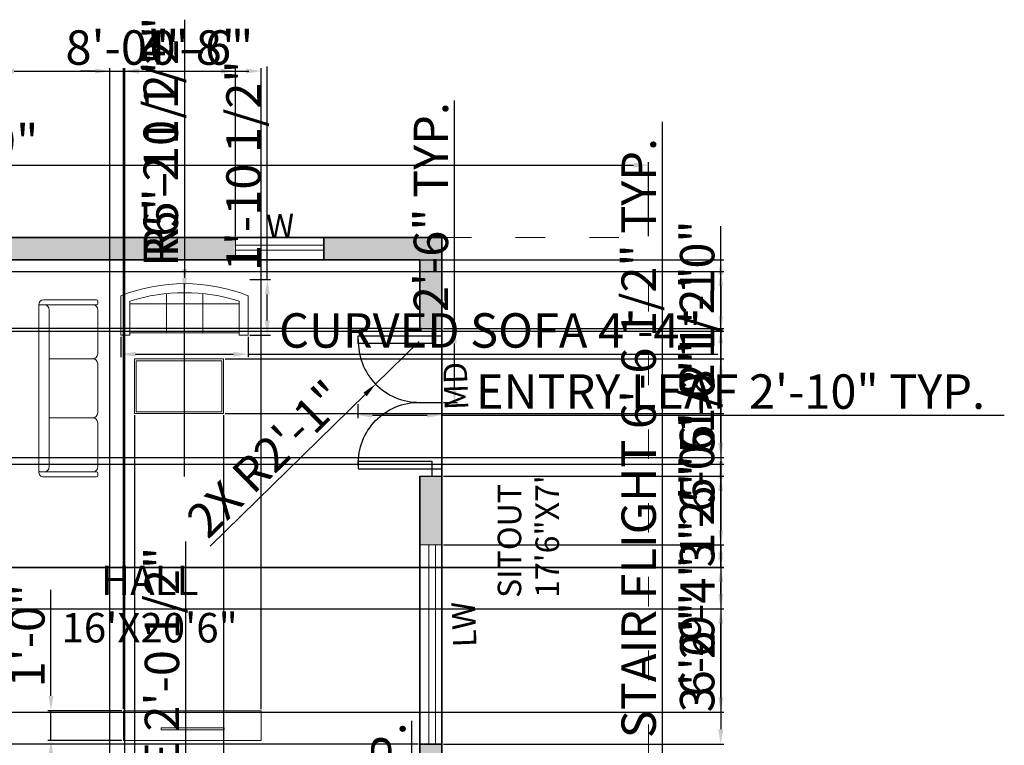
# Model space of a CAD drawing. Units: inches. Extents: x 2961 to 3748, y 1432 to 1961.
# Tile 9 of 9: x 3348 to 3748, y 1658 to 1953. Entities that reach past the tile are written whole.
import ezdxf
from ezdxf.enums import TextEntityAlignment as Align

# ---------------------------------------------------------------- set-up
doc = ezdxf.new("R2010")
doc.units = ezdxf.units.IN
doc.linetypes.add('ACAD_ISO03W100', pattern=[30, 12, -18])
for name, color, linetype, lineweight in [('A-ANNO-DIMS', 2, 'Continuous', 18), ('A-ANNO-TEXT', 7, 'Continuous', 18), ('A-AREA-IDEN', 7, 'Continuous', 18), ('A-DOOR', 3, 'Continuous', 25), ('A-FURN', 8, 'Continuous', 18), ('A-GLAZ', 4, 'Continuous', 18), ('A-ROOF-OVHD', 8, 'ACAD_ISO03W100', 18), ('A-WALL', 7, 'Continuous', 35), ('A-WALL-PATT', 252, 'Continuous', 13)]:
    doc.layers.add(name, color=color, linetype=linetype, lineweight=lineweight)
doc.styles.get("Standard").update_dxf_attribs({"font": 'arial.ttf'})
doc.dimstyles.new('ISO-25', dxfattribs={"dimtxt": 14, "dimasz": 6, "dimexe": 1.25, "dimexo": 0.625, "dimtad": 1, "dimlunit": 3, "dimtxsty": 'Standard', "dimcen": 2.5, "dimadec": 0, "dimazin": 0, "dimtfac": 1, "dimtmove": 0, "dimatfit": 3, "dimfxl": 1, "dimarcsym": 0})

# ---------------------------------------------------------------- blocks, each defined once
blk = doc.blocks.new('sofa')
for p, q in [((1024.17, 311.16), (1024.17, 289.66)), ((1024.67, 311.66), (1025.67, 311.66)), ((1026.17, 308), (1026.17, 311.16)), ((1048.17, 309.66), (1048.17, 291.87)), ((1048.17, 309.66), (1048.17, 309.66)), ((1050.17, 311.66), (1070.17, 311.66)), ((1072.17, 309.66), (1072.17, 291.87)), ((1072.17, 309.66), (1072.17, 309.66)), ((1094.17, 309.66), (1094.17, 311.16)), ((1095.67, 311.66), (1094.67, 311.66)), ((1096.17, 289.66), (1096.17, 311.16)), ((1026.17, 287.66), (1094.17, 287.66))]:
    blk.add_line(p, q)
for points in [[(1046.17, 311.66), (1028.17, 311.66, 0.414214), (1026.17, 309.66), (1026.17, 288.16)], [(1074.17, 311.66), (1092.17, 311.66, -0.414214), (1094.17, 309.66), (1094.17, 288.16)]]:
    blk.add_lwpolyline(points, format="xyb")
blk.add_lwpolyline([(1026.67, 287.66), (1093.67, 287.66, 0.414214), (1094.17, 288.16), (1094.17, 289.87, 0.414214), (1092.17, 291.87), (1028.17, 291.87, 0.414214), (1026.17, 289.87), (1026.17, 288.16, 0.414214)], format="xyb", close=True)
for centre, radius, start, end in [((1024.67, 311.16), 0.5, 90, 180), ((1025.67, 311.16), 0.5, 0, 90), ((1046.17, 309.66), 2, 0, 90), ((1050.17, 309.66), 2, 90, 180), ((1070.17, 309.66), 2, 0, 90), ((1074.17, 309.66), 2, 90, 180), ((1094.67, 311.16), 0.5, 90, 180), ((1095.67, 311.16), 0.5, 0, 90), ((1026.17, 289.66), 2, 180, 270), ((1094.17, 289.66), 2, 270, 0)]:
    blk.add_arc(centre, radius, start, end)
blk = doc.blocks.new('Sofa - Roundback 7 ft.')
for p, q in [((-36.000027, -34), (-36.000027, -11.4696)), ((-12.00002, -32.4421), (-12.00003, -6.5971)), ((11.99997, -32.4421), (11.99998, -6.5971)), ((35.99998, -34), (35.99998, -11.4696)), ((-35.999844, -13.3819), (35.9998, -13.3819)), ((-36.000027, -32.4421), (35.99998, -32.4421))]:
    blk.add_line(p, q)
for points in [[(-36.000027, -34), (-42.000027, -34), (-42.000027, -8)], [(41.99998, -8), (41.99998, -34), (35.99998, -34)]]:
    blk.add_lwpolyline(points)
for centre, radius, start, end in [((0, -114.25), 114.25, 68.43141, 111.5686), ((-0.00001, -127.1968), 121.1968, 72.72033, 107.2797)]:
    blk.add_arc(centre, radius, start, end)
blk = doc.blocks.new('*D14')
at = {"layer": 'A-ANNO-DIMS', "color": 0, "lineweight": -2, "transparency": 16777216}
for p, q in [((3054.27, 1865.26), (3054.27, 1895.31)), ((3603.27, 1865.26), (3603.27, 1895.31)), ((3060.27, 1894.06), (3597.27, 1894.06))]:
    blk.add_line(p, q, dxfattribs=at)
at = {"layer": 'A-ANNO-DIMS', "color": 0, "transparency": 16777216}
for points in [[(3060.27, 1895.06), (3060.27, 1893.06), (3054.27, 1894.06)], [(3597.27, 1895.06), (3597.27, 1893.06), (3603.27, 1894.06)]]:
    blk.add_solid(points, dxfattribs=at)
at = {"layer": 'Defpoints', "color": 0, "transparency": 16777216}
for p in [(3603.27, 1894.06), (3054.27, 1864.64), (3603.27, 1864.64)]:
    blk.add_point(p, dxfattribs=at)
at = {"layer": 'A-ANNO-DIMS', "color": 0, "transparency": 16777216, "insert": (3328.77, 1901.84), "char_height": 14, "attachment_point": 5}
blk.add_mtext('45\'-9"', dxfattribs=at)
blk = doc.blocks.new('WIN-36IN')
for p, q in [((0, 6), (36, 6)), ((0, 3.9), (36, 3.9))]:
    blk.add_line(p, q)
blk.add_lwpolyline([(36, 9), (0, 9), (0, 0), (36, 0)], close=True)
blk = doc.blocks.new('DOOR-ENTRY-LEAF-30IN')
for p, q in [((25, 30), (34, 30)), ((30, 30), (30, 27)), ((30, 27), (34, 27))]:
    blk.add_line(p, q)
blk.add_lwpolyline([(30, 27), (30, 24), (0, 24), (0, 27)], close=True)
blk.add_arc((24.74, 24.75), 24.75, 178.2636, 270.6019)
blk = doc.blocks.new('*D32')
at = {"layer": 'A-ANNO-DIMS', "color": 0, "lineweight": -2, "transparency": 16777216}
for p, q in [((3485.06, 1796.94), (3485.06, 1791.19)), ((3519.27, 1796.94), (3519.27, 1791.19)), ((3491.06, 1792.44), (3513.27, 1792.44)), ((3519.27, 1792.44), (3748.06, 1792.44))]:
    blk.add_line(p, q, dxfattribs=at)
at = {"layer": 'A-ANNO-DIMS', "color": 0, "transparency": 16777216}
for points in [[(3491.06, 1793.44), (3491.06, 1791.44), (3485.06, 1792.44)], [(3513.27, 1793.44), (3513.27, 1791.44), (3519.27, 1792.44)]]:
    blk.add_solid(points, dxfattribs=at)
at = {"layer": 'Defpoints', "color": 0, "transparency": 16777216}
for p in [(3485.06, 1797.57), (3519.27, 1797.57), (3519.27, 1792.44)]:
    blk.add_point(p, dxfattribs=at)
at = {"layer": 'A-ANNO-DIMS', "color": 0, "transparency": 16777216, "insert": (3636.66, 1800.21), "char_height": 14, "attachment_point": 5}
blk.add_mtext('ENTRY LEAF 2\'-10" TYP.', dxfattribs=at)
blk = doc.blocks.new('*D33')
at = {"layer": 'A-ANNO-DIMS', "color": 0, "lineweight": -2, "transparency": 16777216}
for p, q in [((3524.4, 1827.64), (3524.4, 1920.46)), ((3519.89, 1827.64), (3525.65, 1827.64)), ((3524.4, 1803.57), (3524.4, 1821.64)), ((3519.89, 1797.57), (3525.65, 1797.57))]:
    blk.add_line(p, q, dxfattribs=at)
at = {"layer": 'A-ANNO-DIMS', "color": 0, "transparency": 16777216}
for points in [[(3523.4, 1821.64), (3525.4, 1821.64), (3524.4, 1827.64)], [(3523.4, 1803.57), (3525.4, 1803.57), (3524.4, 1797.57)]]:
    blk.add_solid(points, dxfattribs=at)
at = {"layer": 'Defpoints', "color": 0, "transparency": 16777216}
for p in [(3519.27, 1827.64), (3524.4, 1827.64), (3519.27, 1797.57)]:
    blk.add_point(p, dxfattribs=at)
at = {"layer": 'A-ANNO-DIMS', "color": 0, "transparency": 16777216, "insert": (3516.62, 1877.05), "char_height": 14, "attachment_point": 5, "rotation": 90}
blk.add_mtext('2\'-6" TYP.', dxfattribs=at)
blk = doc.blocks.new('*D35')
at = {"layer": 'A-ANNO-DIMS', "color": 0, "lineweight": -2, "transparency": 16777216}
for p, q in [((3507, 1575.49), (3507, 1668.08)), ((3506.23, 1569.49), (3508.25, 1569.49)), ((3507, 1560.25), (3507, 1569.49)), ((3506.23, 1560.25), (3508.25, 1560.25)), ((3507, 1554.25), (3507, 1548.25))]:
    blk.add_line(p, q, dxfattribs=at)
at = {"layer": 'A-ANNO-DIMS', "color": 0, "transparency": 16777216}
for points in [[(3506, 1575.49), (3508, 1575.49), (3507, 1569.49)], [(3506, 1554.25), (3508, 1554.25), (3507, 1560.25)]]:
    blk.add_solid(points, dxfattribs=at)
at = {"layer": 'Defpoints', "color": 0, "transparency": 16777216}
for p in [(3505.61, 1569.49), (3507, 1569.49), (3505.61, 1560.25)]:
    blk.add_point(p, dxfattribs=at)
at = {"layer": 'A-ANNO-DIMS', "color": 0, "transparency": 16777216, "insert": (3499.22, 1624.78), "char_height": 14, "attachment_point": 5, "rotation": 90}
blk.add_mtext('0\'-9" TYP.', dxfattribs=at)
blk = doc.blocks.new('*D36')
at = {"layer": 'A-ANNO-DIMS', "color": 0, "lineweight": -2, "transparency": 16777216}
for p, q in [((3609.01, 1648.54), (3609.01, 1911.68)), ((3597.89, 1648.54), (3610.26, 1648.54)), ((3609.01, 1576.24), (3609.01, 1642.54)), ((3597.89, 1570.24), (3610.26, 1570.24))]:
    blk.add_line(p, q, dxfattribs=at)
at = {"layer": 'A-ANNO-DIMS', "color": 0, "transparency": 16777216}
for points in [[(3608.01, 1642.54), (3610.01, 1642.54), (3609.01, 1648.54)], [(3608.01, 1576.24), (3610.01, 1576.24), (3609.01, 1570.24)]]:
    blk.add_solid(points, dxfattribs=at)
at = {"layer": 'Defpoints', "color": 0, "transparency": 16777216}
for p in [(3597.27, 1648.54), (3609.01, 1648.54), (3597.27, 1570.24)]:
    blk.add_point(p, dxfattribs=at)
at = {"layer": 'A-ANNO-DIMS', "color": 0, "transparency": 16777216, "insert": (3601.15, 1783.11), "char_height": 14, "attachment_point": 5, "rotation": 90}
blk.add_mtext('STAIR FLIGHT 6\'-6 1/2" TYP.', dxfattribs=at)
blk = doc.blocks.new('*D40')
at = {"layer": 'A-ANNO-DIMS', "color": 0, "lineweight": -2, "transparency": 16777216}
for p, q in [((3415.09, 1585.45), (3415.09, 1741.07)), ((3412.07, 1585.45), (3416.34, 1585.45)), ((3415.09, 1567.11), (3415.09, 1579.45)), ((3412.07, 1561.11), (3416.34, 1561.11))]:
    blk.add_line(p, q, dxfattribs=at)
at = {"layer": 'A-ANNO-DIMS', "color": 0, "transparency": 16777216}
for points in [[(3414.09, 1579.45), (3416.09, 1579.45), (3415.09, 1585.45)], [(3414.09, 1567.11), (3416.09, 1567.11), (3415.09, 1561.11)]]:
    blk.add_solid(points, dxfattribs=at)
at = {"layer": 'Defpoints', "color": 0, "transparency": 16777216}
for p in [(3411.44, 1585.45), (3415.09, 1585.45), (3411.44, 1561.11)]:
    blk.add_point(p, dxfattribs=at)
at = {"layer": 'A-ANNO-DIMS', "color": 0, "transparency": 16777216, "insert": (3407.23, 1666.26), "char_height": 14, "attachment_point": 5, "rotation": 90}
blk.add_mtext('FRIDGE 2\'-0 1/2"', dxfattribs=at)
blk = doc.blocks.new('*D48')
at = {"layer": 'A-ANNO-DIMS', "color": 0, "lineweight": -2, "transparency": 16777216}
for p, q in [((3388.72, 1824.34), (3388.72, 1815.95)), ((3440.5, 1824.34), (3440.5, 1815.95)), ((3394.72, 1817.2), (3434.5, 1817.2)), ((3440.5, 1817.2), (3631.5, 1817.2))]:
    blk.add_line(p, q, dxfattribs=at)
at = {"layer": 'A-ANNO-DIMS', "color": 0, "transparency": 16777216}
for points in [[(3394.72, 1818.2), (3394.72, 1816.2), (3388.72, 1817.2)], [(3434.5, 1818.2), (3434.5, 1816.2), (3440.5, 1817.2)]]:
    blk.add_solid(points, dxfattribs=at)
at = {"layer": 'Defpoints', "color": 0, "transparency": 16777216}
for p in [(3388.72, 1824.96), (3440.5, 1824.96), (3440.5, 1817.2)]:
    blk.add_point(p, dxfattribs=at)
at = {"layer": 'A-ANNO-DIMS', "color": 0, "transparency": 16777216, "insert": (3539, 1825.07), "char_height": 14, "attachment_point": 5}
blk.add_mtext('CURVED SOFA 4\'-4"', dxfattribs=at)
blk = doc.blocks.new('*D49')
at = {"layer": 'A-ANNO-DIMS', "color": 0, "lineweight": -2, "transparency": 16777216}
for p, q in [((3448.26, 1847.57), (3448.26, 1934.21)), ((3441.12, 1847.57), (3449.51, 1847.57)), ((3448.26, 1830.96), (3448.26, 1841.57)), ((3441.12, 1824.96), (3449.51, 1824.96))]:
    blk.add_line(p, q, dxfattribs=at)
at = {"layer": 'A-ANNO-DIMS', "color": 0, "transparency": 16777216}
for points in [[(3447.26, 1841.57), (3449.26, 1841.57), (3448.26, 1847.57)], [(3447.26, 1830.96), (3449.26, 1830.96), (3448.26, 1824.96)]]:
    blk.add_solid(points, dxfattribs=at)
at = {"layer": 'Defpoints', "color": 0, "transparency": 16777216}
for p in [(3440.5, 1847.57), (3448.26, 1847.57), (3440.5, 1824.96)]:
    blk.add_point(p, dxfattribs=at)
at = {"layer": 'A-ANNO-DIMS', "color": 0, "transparency": 16777216, "insert": (3440.4, 1893.89), "char_height": 14, "attachment_point": 5, "rotation": 90}
blk.add_mtext('1\'-10 1/2"', dxfattribs=at)
blk = doc.blocks.new('*D52')
at = {"layer": 'A-ANNO-DIMS', "color": 0, "lineweight": -2, "transparency": 16777216}
for p, q in [((3360.27, 1678.21), (3360.27, 1721.36)), ((3389.1, 1672.21), (3359.02, 1672.21)), ((3360.27, 1660.05), (3360.27, 1672.21)), ((3389.1, 1660.05), (3359.02, 1660.05)), ((3360.27, 1654.05), (3360.27, 1648.05))]:
    blk.add_line(p, q, dxfattribs=at)
at = {"layer": 'A-ANNO-DIMS', "color": 0, "transparency": 16777216}
for points in [[(3359.27, 1678.21), (3361.27, 1678.21), (3360.27, 1672.21)], [(3359.27, 1654.05), (3361.27, 1654.05), (3360.27, 1660.05)]]:
    blk.add_solid(points, dxfattribs=at)
at = {"layer": 'Defpoints', "color": 0, "transparency": 16777216}
for p in [(3360.27, 1672.21), (3389.72, 1672.21), (3389.72, 1660.05)]:
    blk.add_point(p, dxfattribs=at)
at = {"layer": 'A-ANNO-DIMS', "color": 0, "transparency": 16777216, "insert": (3352.5, 1702.78), "char_height": 14, "attachment_point": 5, "rotation": 90}
blk.add_mtext('1\'-0"', dxfattribs=at)
blk = doc.blocks.new('*D55')
at = {"layer": 'A-ANNO-DIMS', "color": 0, "lineweight": -2, "transparency": 16777216}
for p, q in [((3339.27, 1865.26), (3339.27, 1933.63)), ((3345.27, 1932.38), (3429.27, 1932.38)), ((3435.27, 1865.26), (3435.27, 1933.63))]:
    blk.add_line(p, q, dxfattribs=at)
at = {"layer": 'A-ANNO-DIMS', "color": 0, "transparency": 16777216}
for points in [[(3345.27, 1933.38), (3345.27, 1931.38), (3339.27, 1932.38)], [(3429.27, 1933.38), (3429.27, 1931.38), (3435.27, 1932.38)]]:
    blk.add_solid(points, dxfattribs=at)
at = {"layer": 'Defpoints', "color": 0, "transparency": 16777216}
for p in [(3435.27, 1932.38), (3339.27, 1864.64), (3435.27, 1864.64)]:
    blk.add_point(p, dxfattribs=at)
at = {"layer": 'A-ANNO-DIMS', "color": 0, "transparency": 16777216, "insert": (3387.27, 1940.15), "char_height": 14, "attachment_point": 5}
blk.add_mtext('8\'-0"', dxfattribs=at)
blk = doc.blocks.new('*D64')
at = {"layer": 'A-ANNO-DIMS', "color": 0, "lineweight": -2, "transparency": 16777216}
for p, q in [((3509.64, 1855.64), (3023.57, 1855.64)), ((3024.82, 1849.64), (3024.82, 1833.64)), ((3509.64, 1827.64), (3023.57, 1827.64)), ((3024.82, 1827.64), (3024.82, 1782.93))]:
    blk.add_line(p, q, dxfattribs=at)
at = {"layer": 'A-ANNO-DIMS', "color": 0, "transparency": 16777216}
for points in [[(3023.82, 1849.64), (3025.82, 1849.64), (3024.82, 1855.64)], [(3023.82, 1833.64), (3025.82, 1833.64), (3024.82, 1827.64)]]:
    blk.add_solid(points, dxfattribs=at)
at = {"layer": 'Defpoints', "color": 0, "transparency": 16777216}
for p in [(3510.27, 1855.64), (3024.82, 1827.64), (3510.27, 1827.64)]:
    blk.add_point(p, dxfattribs=at)
at = {"layer": 'A-ANNO-DIMS', "color": 0, "transparency": 16777216, "insert": (3017.16, 1802.29), "char_height": 14, "attachment_point": 5, "rotation": 90}
blk.add_mtext('2\'-4"', dxfattribs=at)
blk = doc.blocks.new('*D65')
at = {"layer": 'A-ANNO-DIMS', "color": 0, "lineweight": -2, "transparency": 16777216}
for p, q in [((3519.89, 1827.64), (3633.97, 1827.64)), ((3632.72, 1821.64), (3632.72, 1773.64)), ((3519.89, 1767.64), (3633.97, 1767.64))]:
    blk.add_line(p, q, dxfattribs=at)
at = {"layer": 'A-ANNO-DIMS', "color": 0, "transparency": 16777216}
for points in [[(3631.72, 1821.64), (3633.72, 1821.64), (3632.72, 1827.64)], [(3631.72, 1773.64), (3633.72, 1773.64), (3632.72, 1767.64)]]:
    blk.add_solid(points, dxfattribs=at)
at = {"layer": 'Defpoints', "color": 0, "transparency": 16777216}
for p in [(3519.27, 1827.64), (3519.27, 1767.64), (3632.72, 1767.64)]:
    blk.add_point(p, dxfattribs=at)
at = {"layer": 'A-ANNO-DIMS', "color": 0, "transparency": 16777216, "insert": (3624.94, 1797.64), "char_height": 14, "attachment_point": 5, "rotation": 90}
blk.add_mtext('5\'-0"', dxfattribs=at)
blk = doc.blocks.new('*D66')
at = {"layer": 'A-ANNO-DIMS', "color": 0, "lineweight": -2, "transparency": 16777216}
for p, q in [((3519.89, 1767.64), (3633.97, 1767.64)), ((3632.72, 1761.64), (3632.72, 1745.64)), ((3519.89, 1739.64), (3633.97, 1739.64)), ((3632.72, 1739.64), (3632.72, 1694.93))]:
    blk.add_line(p, q, dxfattribs=at)
at = {"layer": 'A-ANNO-DIMS', "color": 0, "transparency": 16777216}
for points in [[(3631.72, 1761.64), (3633.72, 1761.64), (3632.72, 1767.64)], [(3631.72, 1745.64), (3633.72, 1745.64), (3632.72, 1739.64)]]:
    blk.add_solid(points, dxfattribs=at)
at = {"layer": 'Defpoints', "color": 0, "transparency": 16777216}
for p in [(3519.27, 1767.64), (3519.27, 1739.64), (3632.72, 1739.64)]:
    blk.add_point(p, dxfattribs=at)
at = {"layer": 'A-ANNO-DIMS', "color": 0, "transparency": 16777216, "insert": (3625.06, 1714.29), "char_height": 14, "attachment_point": 5, "rotation": 90}
blk.add_mtext('2\'-4"', dxfattribs=at)
blk = doc.blocks.new('*D67')
at = {"layer": 'A-ANNO-DIMS', "color": 0, "lineweight": -2, "transparency": 16777216}
for p, q in [((3519.89, 1739.64), (3633.97, 1739.64)), ((3632.72, 1733.64), (3632.72, 1664.64)), ((3519.89, 1658.64), (3633.97, 1658.64))]:
    blk.add_line(p, q, dxfattribs=at)
at = {"layer": 'A-ANNO-DIMS', "color": 0, "transparency": 16777216}
for points in [[(3631.72, 1733.64), (3633.72, 1733.64), (3632.72, 1739.64)], [(3631.72, 1664.64), (3633.72, 1664.64), (3632.72, 1658.64)]]:
    blk.add_solid(points, dxfattribs=at)
at = {"layer": 'Defpoints', "color": 0, "transparency": 16777216}
for p in [(3519.27, 1739.64), (3519.27, 1658.64), (3632.72, 1658.64)]:
    blk.add_point(p, dxfattribs=at)
at = {"layer": 'A-ANNO-DIMS', "color": 0, "transparency": 16777216, "insert": (3624.94, 1699.14), "char_height": 14, "attachment_point": 5, "rotation": 90}
blk.add_mtext('6\'-9"', dxfattribs=at)
blk = doc.blocks.new('*D68')
at = {"layer": 'A-ANNO-DIMS', "color": 0, "lineweight": -2, "transparency": 16777216}
for p, q in [((3024.82, 1658.64), (3024.82, 1701.79)), ((3509.64, 1658.64), (3023.57, 1658.64)), ((3024.82, 1647.64), (3024.82, 1652.64)), ((3509.64, 1641.64), (3023.57, 1641.64))]:
    blk.add_line(p, q, dxfattribs=at)
at = {"layer": 'A-ANNO-DIMS', "color": 0, "transparency": 16777216}
for points in [[(3023.82, 1652.64), (3025.82, 1652.64), (3024.82, 1658.64)], [(3023.82, 1647.64), (3025.82, 1647.64), (3024.82, 1641.64)]]:
    blk.add_solid(points, dxfattribs=at)
at = {"layer": 'Defpoints', "color": 0, "transparency": 16777216}
for p in [(3024.82, 1658.64), (3510.27, 1658.64), (3510.27, 1641.64)]:
    blk.add_point(p, dxfattribs=at)
at = {"layer": 'A-ANNO-DIMS', "color": 0, "transparency": 16777216, "insert": (3017.04, 1683.21), "char_height": 14, "attachment_point": 5, "rotation": 90}
blk.add_mtext('1\'-5"', dxfattribs=at)
blk = doc.blocks.new('*D70')
at = {"layer": 'A-ANNO-DIMS', "color": 0, "lineweight": -2, "transparency": 16777216}
for p, q in [((3024.82, 1641.64), (3024.82, 1686.09)), ((3383.64, 1641.64), (3023.57, 1641.64)), ((3024.82, 1611.64), (3024.82, 1635.64)), ((3383.64, 1605.64), (3023.57, 1605.64))]:
    blk.add_line(p, q, dxfattribs=at)
at = {"layer": 'A-ANNO-DIMS', "color": 0, "transparency": 16777216}
for points in [[(3023.82, 1635.64), (3025.82, 1635.64), (3024.82, 1641.64)], [(3023.82, 1611.64), (3025.82, 1611.64), (3024.82, 1605.64)]]:
    blk.add_solid(points, dxfattribs=at)
at = {"layer": 'Defpoints', "color": 0, "transparency": 16777216}
for p in [(3024.82, 1641.64), (3384.27, 1641.64), (3384.27, 1605.64)]:
    blk.add_point(p, dxfattribs=at)
at = {"layer": 'A-ANNO-DIMS', "color": 0, "transparency": 16777216, "insert": (3017.04, 1666.87), "char_height": 14, "attachment_point": 5, "rotation": 90}
blk.add_mtext('3\'-0"', dxfattribs=at)
blk = doc.blocks.new('*D71')
at = {"layer": 'A-ANNO-DIMS', "color": 0, "lineweight": -2, "transparency": 16777216}
for p, q in [((3255.89, 1772.53), (3633.97, 1772.53)), ((3632.72, 1736.64), (3632.72, 1766.53)), ((3255.89, 1730.64), (3633.97, 1730.64))]:
    blk.add_line(p, q, dxfattribs=at)
at = {"layer": 'A-ANNO-DIMS', "color": 0, "transparency": 16777216}
for points in [[(3631.72, 1766.53), (3633.72, 1766.53), (3632.72, 1772.53)], [(3631.72, 1736.64), (3633.72, 1736.64), (3632.72, 1730.64)]]:
    blk.add_solid(points, dxfattribs=at)
at = {"layer": 'Defpoints', "color": 0, "transparency": 16777216}
for p in [(3255.27, 1772.53), (3632.72, 1772.53), (3255.27, 1730.64)]:
    blk.add_point(p, dxfattribs=at)
at = {"layer": 'A-ANNO-DIMS', "color": 0, "transparency": 16777216, "insert": (3624.94, 1751.59), "char_height": 14, "attachment_point": 5, "rotation": 90}
blk.add_mtext('3\'-6"', dxfattribs=at)
blk = doc.blocks.new('*D72')
at = {"layer": 'A-ANNO-DIMS', "color": 0, "lineweight": -2, "transparency": 16777216}
for p, q in [((3255.89, 1713.64), (3633.97, 1713.64)), ((3632.72, 1677.64), (3632.72, 1707.64)), ((3255.89, 1671.64), (3633.97, 1671.64))]:
    blk.add_line(p, q, dxfattribs=at)
at = {"layer": 'A-ANNO-DIMS', "color": 0, "transparency": 16777216}
for points in [[(3631.72, 1707.64), (3633.72, 1707.64), (3632.72, 1713.64)], [(3631.72, 1677.64), (3633.72, 1677.64), (3632.72, 1671.64)]]:
    blk.add_solid(points, dxfattribs=at)
at = {"layer": 'Defpoints', "color": 0, "transparency": 16777216}
for p in [(3255.27, 1713.64), (3632.72, 1713.64), (3255.27, 1671.64)]:
    blk.add_point(p, dxfattribs=at)
at = {"layer": 'A-ANNO-DIMS', "color": 0, "transparency": 16777216, "insert": (3624.94, 1692.64), "char_height": 14, "attachment_point": 5, "rotation": 90}
blk.add_mtext('3\'-6"', dxfattribs=at)
blk = doc.blocks.new('*D76')
at = {"layer": 'A-ANNO-DIMS', "color": 0, "lineweight": -2, "transparency": 16777216}
for p, q in [((3632.72, 1730.53), (3632.72, 1773.68)), ((3264.89, 1730.53), (3633.97, 1730.53)), ((3632.72, 1719.64), (3632.72, 1724.53)), ((3264.89, 1713.64), (3633.97, 1713.64))]:
    blk.add_line(p, q, dxfattribs=at)
at = {"layer": 'A-ANNO-DIMS', "color": 0, "transparency": 16777216}
for points in [[(3631.72, 1724.53), (3633.72, 1724.53), (3632.72, 1730.53)], [(3631.72, 1719.64), (3633.72, 1719.64), (3632.72, 1713.64)]]:
    blk.add_solid(points, dxfattribs=at)
at = {"layer": 'Defpoints', "color": 0, "transparency": 16777216}
for p in [(3264.27, 1730.53), (3632.72, 1730.53), (3264.27, 1713.64)]:
    blk.add_point(p, dxfattribs=at)
at = {"layer": 'A-ANNO-DIMS', "color": 0, "transparency": 16777216, "insert": (3624.94, 1755.11), "char_height": 14, "attachment_point": 5, "rotation": 90}
blk.add_mtext('1\'-5"', dxfattribs=at)
blk = doc.blocks.new('*D78')
at = {"layer": 'A-ANNO-DIMS', "color": 0, "lineweight": -2, "transparency": 16777216}
for p, q in [((3394.23, 1792.44), (3394.23, 1473.94)), ((3430.5, 1792.44), (3430.5, 1473.94)), ((3400.23, 1475.19), (3424.5, 1475.19)), ((3430.5, 1475.19), (3507.58, 1475.19))]:
    blk.add_line(p, q, dxfattribs=at)
at = {"layer": 'A-ANNO-DIMS', "color": 0, "transparency": 16777216}
for points in [[(3400.23, 1476.19), (3400.23, 1474.19), (3394.23, 1475.19)], [(3424.5, 1476.19), (3424.5, 1474.19), (3430.5, 1475.19)]]:
    blk.add_solid(points, dxfattribs=at)
at = {"layer": 'Defpoints', "color": 0, "transparency": 16777216}
for p in [(3394.23, 1793.06), (3430.5, 1793.06), (3430.5, 1475.19)]:
    blk.add_point(p, dxfattribs=at)
at = {"layer": 'A-ANNO-DIMS', "color": 0, "transparency": 16777216, "insert": (3472.04, 1483.06), "char_height": 14, "attachment_point": 5}
blk.add_mtext('3\'-0 1/2"', dxfattribs=at)
blk = doc.blocks.new('*D79')
at = {"layer": 'A-ANNO-DIMS', "color": 0, "lineweight": -2, "transparency": 16777216}
for p, q in [((3632.72, 1815.29), (3632.72, 1869.31)), ((3431.13, 1815.29), (3633.97, 1815.29)), ((3632.72, 1799.06), (3632.72, 1809.29)), ((3431.13, 1793.06), (3633.97, 1793.06))]:
    blk.add_line(p, q, dxfattribs=at)
at = {"layer": 'A-ANNO-DIMS', "color": 0, "transparency": 16777216}
for points in [[(3631.72, 1809.29), (3633.72, 1809.29), (3632.72, 1815.29)], [(3631.72, 1799.06), (3633.72, 1799.06), (3632.72, 1793.06)]]:
    blk.add_solid(points, dxfattribs=at)
at = {"layer": 'Defpoints', "color": 0, "transparency": 16777216}
for p in [(3430.5, 1815.29), (3632.72, 1815.29), (3430.5, 1793.06)]:
    blk.add_point(p, dxfattribs=at)
at = {"layer": 'A-ANNO-DIMS', "color": 0, "transparency": 16777216, "insert": (3624.94, 1845.3), "char_height": 14, "attachment_point": 5, "rotation": 90}
blk.add_mtext('1\'-10"', dxfattribs=at)
blk = doc.blocks.new('*D80')
at = {"layer": 'A-ANNO-DIMS', "color": 0, "lineweight": -2, "transparency": 16777216}
for p, q in [((3389.72, 1672.83), (3389.72, 1933.63)), ((3395.72, 1932.38), (3439.76, 1932.38)), ((3445.76, 1672.83), (3445.76, 1933.63))]:
    blk.add_line(p, q, dxfattribs=at)
at = {"layer": 'A-ANNO-DIMS', "color": 0, "transparency": 16777216}
for points in [[(3395.72, 1933.38), (3395.72, 1931.38), (3389.72, 1932.38)], [(3439.76, 1933.38), (3439.76, 1931.38), (3445.76, 1932.38)]]:
    blk.add_solid(points, dxfattribs=at)
at = {"layer": 'Defpoints', "color": 0, "transparency": 16777216}
for p in [(3445.76, 1932.38), (3389.72, 1672.21), (3445.76, 1672.21)]:
    blk.add_point(p, dxfattribs=at)
at = {"layer": 'A-ANNO-DIMS', "color": 0, "transparency": 16777216, "insert": (3417.74, 1940.15), "char_height": 14, "attachment_point": 5}
blk.add_mtext('4\'-8"', dxfattribs=at)
blk = doc.blocks.new('*D83')
at = {"layer": 'A-ANNO-DIMS', "color": 0, "lineweight": -2, "transparency": 16777216}
for p, q in [((3123.89, 1855.64), (3633.97, 1855.64)), ((3632.72, 1781.22), (3632.72, 1849.64)), ((3123.89, 1775.22), (3633.97, 1775.22))]:
    blk.add_line(p, q, dxfattribs=at)
at = {"layer": 'A-ANNO-DIMS', "color": 0, "transparency": 16777216}
for points in [[(3631.72, 1849.64), (3633.72, 1849.64), (3632.72, 1855.64)], [(3631.72, 1781.22), (3633.72, 1781.22), (3632.72, 1775.22)]]:
    blk.add_solid(points, dxfattribs=at)
at = {"layer": 'Defpoints', "color": 0, "transparency": 16777216}
for p in [(3123.27, 1855.64), (3632.72, 1855.64), (3123.27, 1775.22)]:
    blk.add_point(p, dxfattribs=at)
at = {"layer": 'A-ANNO-DIMS', "color": 0, "transparency": 16777216, "insert": (3624.85, 1815.43), "char_height": 14, "attachment_point": 5, "rotation": 90}
blk.add_mtext('6\'-8 1/2"', dxfattribs=at)
blk = doc.blocks.new('*D86')
at = {"layer": 'A-ANNO-DIMS', "color": 0, "lineweight": -2, "transparency": 16777216}
for p, q in [((3091.52, 1850.93), (3633.97, 1850.93)), ((3632.72, 1844.93), (3632.72, 1832.66)), ((3082.42, 1826.66), (3633.97, 1826.66)), ((3632.72, 1826.66), (3632.72, 1749.34))]:
    blk.add_line(p, q, dxfattribs=at)
at = {"layer": 'A-ANNO-DIMS', "color": 0, "transparency": 16777216}
for points in [[(3631.72, 1844.93), (3633.72, 1844.93), (3632.72, 1850.93)], [(3631.72, 1832.66), (3633.72, 1832.66), (3632.72, 1826.66)]]:
    blk.add_solid(points, dxfattribs=at)
at = {"layer": 'Defpoints', "color": 0, "transparency": 16777216}
for p in [(3090.9, 1850.93), (3081.8, 1826.66), (3632.72, 1826.66)]:
    blk.add_point(p, dxfattribs=at)
at = {"layer": 'A-ANNO-DIMS', "color": 0, "transparency": 16777216, "insert": (3624.85, 1785), "char_height": 14, "attachment_point": 5, "rotation": 90}
blk.add_mtext('2\'-0 1/2"', dxfattribs=at)
blk = doc.blocks.new('*D87')
at = {"layer": 'A-ANNO-DIMS', "color": 0, "lineweight": -2, "transparency": 16777216}
for p, q in [((3378.27, 1932.38), (3372.27, 1932.38)), ((3384.27, 1514.26), (3384.27, 1933.63)), ((3384.27, 1932.38), (3390.27, 1932.38)), ((3390.27, 1514.26), (3390.27, 1933.63)), ((3396.27, 1932.38), (3440.73, 1932.38))]:
    blk.add_line(p, q, dxfattribs=at)
at = {"layer": 'A-ANNO-DIMS', "color": 0, "transparency": 16777216}
for points in [[(3378.27, 1933.38), (3378.27, 1931.38), (3384.27, 1932.38)], [(3396.27, 1933.38), (3396.27, 1931.38), (3390.27, 1932.38)]]:
    blk.add_solid(points, dxfattribs=at)
at = {"layer": 'Defpoints', "color": 0, "transparency": 16777216}
for p in [(3390.27, 1932.38), (3384.27, 1513.64), (3390.27, 1513.64)]:
    blk.add_point(p, dxfattribs=at)
at = {"layer": 'A-ANNO-DIMS', "color": 0, "transparency": 16777216, "insert": (3421.5, 1940.15), "char_height": 14, "attachment_point": 5}
blk.add_mtext('0\'-6"', dxfattribs=at)
blk = doc.blocks.new('*D91')
at = {"layer": 'A-ANNO-DIMS', "color": 0, "lineweight": -2, "transparency": 16777216}
for p, q in [((3414.61, 1938.71), (3414.61, 1848.22)), ((3414.61, 1767.51), (3414.61, 1842.22))]:
    blk.add_line(p, q, dxfattribs=at)
at = {"layer": 'A-ANNO-DIMS', "color": 0, "transparency": 16777216}
blk.add_solid([(3413.61, 1848.22), (3415.61, 1848.22), (3414.61, 1842.22)], dxfattribs=at)
at = {"layer": 'Defpoints', "color": 0, "transparency": 16777216}
for p in [(3414.61, 1842.22), (3414.61, 1767.51)]:
    blk.add_point(p, dxfattribs=at)
at = {"layer": 'A-ANNO-DIMS', "color": 0, "transparency": 16777216, "insert": (3406.74, 1896.47), "char_height": 14, "attachment_point": 5, "rotation": 90}
blk.add_mtext('R6\'-2 1/2"', dxfattribs=at)
blk = doc.blocks.new('*D92')
at = {"layer": 'A-ANNO-DIMS', "color": 0, "lineweight": -2, "transparency": 16777216}
for p, q in [((3414.61, 1953.29), (3414.61, 1851.92)), ((3414.61, 1775.5), (3414.61, 1845.92))]:
    blk.add_line(p, q, dxfattribs=at)
at = {"layer": 'A-ANNO-DIMS', "color": 0, "transparency": 16777216}
blk.add_solid([(3413.61, 1851.92), (3415.61, 1851.92), (3414.61, 1845.92)], dxfattribs=at)
at = {"layer": 'Defpoints', "color": 0, "transparency": 16777216}
for p in [(3414.61, 1845.92), (3414.61, 1775.5)]:
    blk.add_point(p, dxfattribs=at)
at = {"layer": 'A-ANNO-DIMS', "color": 0, "transparency": 16777216, "insert": (3406.74, 1905.6), "char_height": 14, "attachment_point": 5, "rotation": 90}
blk.add_mtext('R5\'-10 1/2"', dxfattribs=at)
blk = doc.blocks.new('*D96')
at = {"layer": 'A-ANNO-DIMS', "color": 0, "lineweight": -2, "transparency": 16777216}
for p, q in [((3510.01, 1822.39), (3492.33, 1805.06)), ((3425.08, 1739.12), (3488.05, 1800.86))]:
    blk.add_line(p, q, dxfattribs=at)
at = {"layer": 'A-ANNO-DIMS', "color": 0, "transparency": 16777216}
blk.add_solid([(3487.35, 1801.57), (3488.75, 1800.15), (3492.33, 1805.06)], dxfattribs=at)
at = {"layer": 'Defpoints', "color": 0, "transparency": 16777216}
for p in [(3510.01, 1822.39), (3492.33, 1805.06)]:
    blk.add_point(p, dxfattribs=at)
at = {"layer": 'A-ANNO-DIMS', "color": 0, "transparency": 16777216, "insert": (3449.06, 1773.36), "char_height": 14, "attachment_point": 5, "rotation": 44.4334}
blk.add_mtext('2X R2\'-1"', dxfattribs=at)

msp = doc.modelspace()

# ---------------------------------------------------------------- hatches: boundary and pattern name
at = {"layer": 'A-WALL-PATT'}
h = msp.add_hatch(color=256, dxfattribs=at)
h.set_gradient(color1=(41, 49, 137), color2=(41, 49, 137), tint=1)
h.paths.add_polyline_path([(3255.267, 1671.639), (3255.267, 1513.639), (3251.267, 1513.639), (3251.267, 1504.639), (3268.267, 1504.639), (3268.267, 1513.639), (3264.267, 1513.639), (3264.267, 1671.639), (3259.767, 1671.639)])
h.paths.add_polyline_path([(3063.267, 1513.639), (3063.267, 1677.639), (3054.267, 1677.639), (3054.267, 1504.639), (3215.267, 1504.639), (3215.267, 1513.639)])
h.paths.add_polyline_path([(3304.267, 1513.639), (3304.267, 1504.639), (3456.267, 1504.639), (3456.267, 1513.639), (3390.267, 1513.639), (3390.267, 1605.639), (3384.267, 1605.639), (3384.267, 1513.639)])
h.paths.add_polyline_path([(3510.267, 1605.639), (3510.267, 1513.639), (3492.267, 1513.639), (3492.267, 1504.639), (3546.267, 1504.639), (3546.267, 1513.639), (3519.267, 1513.639), (3519.267, 1605.639)])
h.paths.add_polyline_path([(3340.267, 1654.639), (3340.267, 1645.639), (3510.267, 1645.639), (3510.267, 1641.639), (3519.267, 1641.639), (3519.267, 1658.639), (3510.267, 1658.639), (3510.267, 1654.639)])
h.paths.add_polyline_path([(3223.801, 1864.639), (3223.801, 1855.639), (3255.267, 1855.639), (3255.267, 1772.534), (3264.267, 1772.534), (3264.267, 1855.639), (3303.267, 1855.639), (3303.267, 1864.639)])
h.paths.add_polyline_path([(3339.267, 1864.639), (3339.267, 1855.639), (3435.267, 1855.639), (3435.267, 1864.639)])
h.paths.add_polyline_path([(3471.267, 1864.639), (3471.267, 1855.639), (3510.267, 1855.639), (3510.267, 1827.639), (3519.267, 1827.639), (3519.267, 1864.639)])
h.paths.add_polyline_path([(3510.267, 1767.639), (3510.267, 1739.639), (3519.267, 1739.639), (3519.267, 1767.639)])
h.paths.add_polyline_path([(3123.267, 1726.639), (3123.267, 1855.639), (3187.801, 1855.639), (3187.801, 1864.639), (3054.267, 1864.639), (3054.267, 1837.201), (3063.267, 1837.201), (3063.267, 1855.639), (3117.267, 1855.639), (3117.267, 1726.639), (3103.267, 1726.639), (3103.267, 1717.639), (3255.267, 1717.639), (3255.267, 1713.639), (3264.267, 1713.639), (3264.267, 1730.534), (3255.267, 1730.639), (3255.267, 1726.639)])
h.paths.add_polyline_path([(3597.267, 1654.639), (3597.267, 1513.639), (3570.267, 1513.639), (3570.267, 1504.639), (3603.267, 1504.639), (3603.267, 1654.639)])
h.paths.add_polyline_path([(3054.267, 1813.201), (3054.267, 1713.639), (3063.267, 1713.639), (3063.267, 1717.639), (3069.267, 1717.639), (3069.267, 1726.639), (3063.267, 1726.639), (3063.267, 1813.201)], flags=17)

# ---------------------------------------------------------------- linework, layer by layer
at = {"layer": 'A-DOOR'}
msp.add_line((3510.267, 1797.639), (3519.267, 1797.639), dxfattribs=at)
at = {"layer": 'A-FURN'}
for points in [[(3394.234, 1793.062), (3394.234, 1815.286), (3430.505, 1815.286), (3430.505, 1793.062)], [(3394.966, 1793.793), (3394.966, 1814.554), (3429.774, 1814.554), (3429.774, 1793.793)], [(3389.724, 1660.049), (3389.724, 1672.208), (3445.761, 1672.208), (3445.761, 1660.049)], [(3405.044, 1664.403), (3405.044, 1665.182), (3430.713, 1665.182), (3430.713, 1664.403)]]:
    msp.add_lwpolyline(points, close=True, dxfattribs=at)
at = {"layer": 'A-GLAZ'}
for p, q in [((3513.971, 1739.639), (3513.971, 1658.639)), ((3516.623, 1739.639), (3516.623, 1658.639))]:
    msp.add_line(p, q, dxfattribs=at)
msp.add_lwpolyline([(3519.267, 1739.639), (3519.267, 1658.639), (3510.267, 1658.639), (3510.267, 1739.639)], close=True, dxfattribs=at)
at = {"layer": 'A-ROOF-OVHD'}
for p in [(3519.267, 1864.639), (3603.267, 1654.639)]:
    msp.add_line(p, (3603.267, 1864.639), dxfattribs=at)
at = {"layer": 'A-WALL'}
for p, q in [((3054.267, 1864.639), (3519.267, 1864.639)), ((3471.267, 1855.639), (3471.267, 1864.639)), ((3519.267, 1513.639), (3519.267, 1864.639)), ((3510.267, 1855.639), (3264.267, 1855.639)), ((3510.267, 1827.639), (3510.267, 1855.639)), ((3510.267, 1654.639), (3510.267, 1767.639)), ((3510.267, 1658.639), (3519.267, 1658.639))]:
    msp.add_line(p, q, dxfattribs=at)

# ---------------------------------------------------------------- block references
at = {"layer": 'A-DOOR'}
msp.add_blockref('DOOR-ENTRY-LEAF-30IN', (3485.267, 1797.639), dxfattribs=at)
at = {"layer": 'A-DOOR', "extrusion": (0, 0, -1), "zscale": -1, "rotation": 180}
msp.add_blockref('DOOR-ENTRY-LEAF-30IN', (-3485.267, 1797.639), dxfattribs=at)
at = {"layer": 'A-FURN', "xscale": 0.6164332533546721, "yscale": 0.6164332533546721, "zscale": 0.6164332533546721}
msp.add_blockref('Sofa - Roundback 7 ft.', (3414.607, 1845.923), dxfattribs=at)
at = {"layer": 'A-FURN', "rotation": 269.9999999999999}
msp.add_blockref('sofa', (3067.628, 2863.51), dxfattribs=at)
at = {"layer": 'A-GLAZ'}
msp.add_blockref('WIN-36IN', (3435.267, 1855.639), dxfattribs=at)

# ---------------------------------------------------------------- texts
at = {"layer": 'A-ANNO-TEXT'}
for s, height, rotation, p in [('W', 9.571, 2.15165, (3453.762, 1864.639)), ('MD', 9.5707, 92.15165, (3529.698, 1804.461)), ('LW', 9.5707, 92.15165, (3533.06, 1707.464))]:
    msp.add_text(s, height=height, rotation=rotation, dxfattribs=at).set_placement(p, align=Align.CENTER)
at = {"layer": 'A-AREA-IDEN'}
for s, p in [('17\'6"X7\'', (3566.936, 1718.079)), ('SITOUT', (3551.561, 1718.079))]:
    msp.add_text(s, height=9.5707, rotation=90, dxfattribs=at).set_placement(p)
for s, p in [('HALL', (3400.401, 1719.253)), ('16\'X20\'6"', (3400.401, 1699.976))]:
    msp.add_text(s, height=12, dxfattribs=at).set_placement(p, align=Align.CENTER)

# ---------------------------------------------------------------- dimensions: what is measured, and where the dimension line sits
at = {"layer": 'A-ANNO-DIMS'}
for center, mpoint, picture, middle in [((3414.607, 1775.495), (3414.607, 1845.923), '*D92', (3406.743, 1905.604)), ((3414.607, 1767.514), (3414.607, 1842.224), '*D91', (3406.743, 1896.467))]:
    dim = msp.add_radius_dim(center=center, mpoint=mpoint, dimstyle='ISO-25', override={"dimdec": 1, "dimlfac": 1, "dimrnd": 0, "dimzin": 1, "dimdsep": 46, "dimlunit": 4, "dimfrac": 2}, dxfattribs=at)
    dim.commit()
    dim.dimension.update_dxf_attribs({"geometry": picture, "text_midpoint": middle})
for base, p1, p2, override, picture, middle in [((3435.267, 1932.38), (3339.267, 1864.639), (3435.267, 1864.639), {"dimdec": 1, "dimlfac": 1, "dimrnd": 0, "dimzin": 1, "dimdsep": 46, "dimlunit": 4, "dimfrac": 2}, '*D55', (3387.267, 1940.153)), ((3390.267, 1932.38), (3384.267, 1513.639), (3390.267, 1513.639), {"dimdec": 1, "dimlfac": 1, "dimrnd": 0, "dimzin": 1, "dimdsep": 46, "dimlunit": 4, "dimfrac": 2}, '*D87', (3421.5, 1940.153)), ((3445.761, 1932.38), (3389.724, 1672.208), (3445.761, 1672.208), {"dimdec": 1, "dimlfac": 1, "dimrnd": 0, "dimzin": 1, "dimdsep": 46, "dimlunit": 4, "dimfrac": 2}, '*D80', (3417.742, 1940.153)), ((3603.267, 1894.063), (3054.267, 1864.639), (3603.267, 1864.639), {"dimclrd": 0, "dimclre": 0, "dimclrt": 0}, '*D14', (3328.767, 1901.836)), ((3430.505, 1475.189), (3394.234, 1793.062), (3430.505, 1793.062), {"dimdec": 1, "dimlfac": 1, "dimrnd": 0, "dimzin": 1, "dimdsep": 46, "dimlunit": 4, "dimfrac": 2}, '*D78', (3472.044, 1483.057))]:
    dim = msp.add_linear_dim(base=base, p1=p1, p2=p2, dimstyle='ISO-25', override=override, dxfattribs=at)
    dim.commit()
    dim.dimension.update_dxf_attribs({"geometry": picture, "text_midpoint": middle})
for base, p1, p2, picture, middle in [((3448.264, 1847.567), (3440.497, 1824.964), (3440.497, 1847.567), '*D49', (3440.4, 1893.89)), ((3632.717, 1815.286), (3430.505, 1793.062), (3430.505, 1815.286), '*D79', (3624.944, 1845.298)), ((3024.817, 1827.639), (3510.267, 1855.639), (3510.267, 1827.639), '*D64', (3017.163, 1802.287)), ((3632.717, 1855.639), (3123.267, 1775.22), (3123.267, 1855.639), '*D83', (3624.853, 1815.429)), ((3632.717, 1826.664), (3090.897, 1850.93), (3081.797, 1826.664), '*D86', (3624.853, 1785)), ((3632.717, 1767.639), (3519.267, 1827.639), (3519.267, 1767.639), '*D65', (3624.944, 1797.639)), ((3632.717, 1730.534), (3264.267, 1713.639), (3264.266, 1730.534), '*D76', (3624.944, 1755.108)), ((3632.717, 1772.534), (3255.267, 1730.639), (3255.267, 1772.534), '*D71', (3624.939, 1751.587)), ((3632.717, 1739.639), (3519.267, 1767.639), (3519.267, 1739.639), '*D66', (3625.063, 1714.287)), ((3632.717, 1658.639), (3519.267, 1739.639), (3519.267, 1658.639), '*D67', (3624.944, 1699.139)), ((3360.274, 1672.208), (3389.724, 1660.049), (3389.724, 1672.208), '*D52', (3352.501, 1702.782)), ((3632.717, 1713.639), (3255.267, 1671.639), (3255.267, 1713.639), '*D72', (3624.939, 1692.639)), ((3024.817, 1658.639), (3510.267, 1641.639), (3510.267, 1658.639), '*D68', (3017.044, 1683.212)), ((3024.817, 1641.639), (3384.267, 1605.639), (3384.267, 1641.639), '*D70', (3017.039, 1666.867))]:
    dim = msp.add_linear_dim(base=base, p1=p1, p2=p2, angle=90, dimstyle='ISO-25', override={"dimdec": 1, "dimlfac": 1, "dimrnd": 0, "dimzin": 1, "dimdsep": 46, "dimlunit": 4, "dimfrac": 2}, dxfattribs=at)
    dim.commit()
    dim.dimension.update_dxf_attribs({"geometry": picture, "text_midpoint": middle})
for base, p1, p2, text, picture, middle in [((3524.397, 1827.639), (3519.267, 1797.568), (3519.267, 1827.639), '<> TYP.', '*D33', (3516.624, 1877.052)), ((3609.012, 1648.539), (3597.267, 1570.239), (3597.267, 1648.539), 'STAIR FLIGHT <> TYP.', '*D36', (3601.148, 1783.112)), ((3415.091, 1585.45), (3411.44, 1561.114), (3411.44, 1585.45), 'FRIDGE <>', '*D40', (3407.227, 1666.258)), ((3506.995, 1569.49), (3505.609, 1560.247), (3505.609, 1569.49), '<> TYP.', '*D35', (3499.222, 1624.783))]:
    dim = msp.add_linear_dim(base=base, p1=p1, p2=p2, angle=90, text=text, dimstyle='ISO-25', override={"dimdec": 1, "dimlfac": 1, "dimrnd": 0, "dimzin": 1, "dimdsep": 46, "dimlunit": 4, "dimfrac": 2}, dxfattribs=at)
    dim.commit()
    dim.dimension.update_dxf_attribs({"geometry": picture, "text_midpoint": middle})
for base, p1, p2, text, picture, middle in [((3440.497, 1817.197), (3388.717, 1824.964), (3440.497, 1824.964), 'CURVED SOFA <>', '*D48', (3539.001, 1825.066)), ((3519.267, 1792.437), (3485.063, 1797.568), (3519.267, 1797.568), 'ENTRY LEAF <> TYP.', '*D32', (3636.665, 1800.21))]:
    dim = msp.add_linear_dim(base=base, p1=p1, p2=p2, text=text, dimstyle='ISO-25', override={"dimdec": 1, "dimlfac": 1, "dimrnd": 0, "dimzin": 1, "dimdsep": 46, "dimlunit": 4, "dimfrac": 2}, dxfattribs=at)
    dim.commit()
    dim.dimension.update_dxf_attribs({"geometry": picture, "text_midpoint": middle})
dim = msp.add_radius_dim(center=(3510.007, 1822.389), mpoint=(3492.333, 1805.061), text='2X <>', dimstyle='ISO-25', override={"dimdec": 1, "dimlfac": 1, "dimrnd": 0, "dimzin": 1, "dimdsep": 46, "dimlunit": 4, "dimfrac": 2}, dxfattribs=at)
dim.commit()
dim.dimension.update_dxf_attribs({"geometry": '*D96', "text_midpoint": (3449.06, 1773.361)})

doc.saveas('drawing.dxf')
